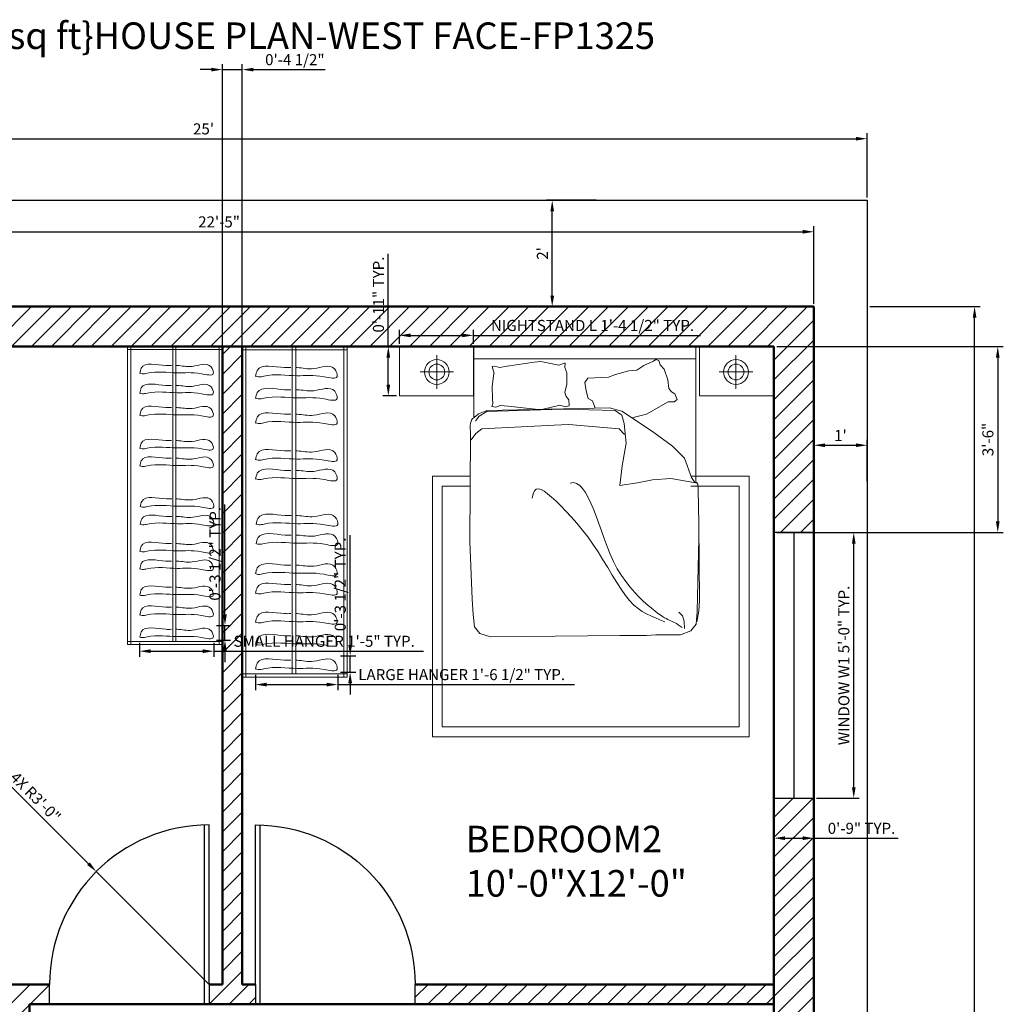
# Model space of a CAD drawing. Units: inches. Extents: x 3542 to 3908, y 2103 to 2666.
# Tile 4 of 4: x 3685 to 3907, y 2444 to 2666. Entities that reach past the tile are written whole.
import ezdxf

# ---------------------------------------------------------------- set-up
doc = ezdxf.new("R2010")
doc.units = ezdxf.units.IN
for name, color, linetype, lineweight in [('A-ANNO-DIMS', 2, 'Continuous', 18), ('A-ANNO-TEXT', 7, 'Continuous', 25), ('A-AREA-IDEN', 7, 'Continuous', 25), ('A-DOOR', 3, 'Continuous', 25), ('A-FLOR-CASE', 8, 'Continuous', 18), ('A-FURN', 8, 'Continuous', 18), ('A-GLAZ', 5, 'Continuous', 25), ('A-WALL', 7, 'Continuous', 50), ('A-WALL-PATT', 252, 'Continuous', 13), ('C-PROP', 7, 'Continuous', 25)]:
    doc.layers.add(name, color=color, linetype=linetype, lineweight=lineweight)
doc.styles.get("Standard").update_dxf_attribs({"font": 'arial.ttf'})
doc.dimstyles.new('ISO-25', dxfattribs={"dimtxt": 2.5, "dimasz": 2.5, "dimexe": 1.25, "dimexo": 0.625, "dimtad": 1, "dimdec": 0, "dimlunit": 3, "dimtxsty": 'Standard', "dimcen": 2.5, "dimadec": 0, "dimazin": 0, "dimtfac": 1, "dimtdec": 0, "dimtmove": 0, "dimatfit": 3, "dimfxl": 1, "dimarcsym": 0})

# ---------------------------------------------------------------- blocks, each defined once
blk = doc.blocks.new('*D5')
at = {"layer": 'A-ANNO-DIMS', "color": 0, "lineweight": -2, "transparency": 16777216}
for p, q in [((3815.51, 2625.48), (3804.33, 2625.48)), ((3805.58, 2603.98), (3805.58, 2622.98)), ((3815.51, 2601.48), (3804.33, 2601.48))]:
    blk.add_line(p, q, dxfattribs=at)
at = {"layer": 'A-ANNO-DIMS', "color": 0, "transparency": 16777216}
for points in [[(3805.17, 2622.98), (3806, 2622.98), (3805.58, 2625.48)], [(3805.17, 2603.98), (3806, 2603.98), (3805.58, 2601.48)]]:
    blk.add_solid(points, dxfattribs=at)
at = {"layer": 'Defpoints', "color": 0, "transparency": 16777216}
for p in [(3805.58, 2625.48), (3816.14, 2625.48), (3816.14, 2601.48)]:
    blk.add_point(p, dxfattribs=at)
at = {"layer": 'A-ANNO-DIMS', "color": 0, "transparency": 16777216, "insert": (3803.7, 2613.48), "char_height": 2.5, "attachment_point": 5, "rotation": 90}
blk.add_mtext("2'", dxfattribs=at)
blk = doc.blocks.new('*D6')
at = {"layer": 'A-ANNO-DIMS', "color": 0, "lineweight": -2, "transparency": 16777216}
for p, q in [((3864.64, 2562.06), (3864.64, 2571.43)), ((3867.14, 2570.18), (3874.14, 2570.18)), ((3876.64, 2562.06), (3876.64, 2571.43))]:
    blk.add_line(p, q, dxfattribs=at)
at = {"layer": 'A-ANNO-DIMS', "color": 0, "transparency": 16777216}
for points in [[(3867.14, 2570.6), (3867.14, 2569.77), (3864.64, 2570.18)], [(3874.14, 2570.6), (3874.14, 2569.77), (3876.64, 2570.18)]]:
    blk.add_solid(points, dxfattribs=at)
at = {"layer": 'Defpoints', "color": 0, "transparency": 16777216}
for p in [(3876.64, 2570.18), (3864.64, 2561.44), (3876.64, 2561.44)]:
    blk.add_point(p, dxfattribs=at)
at = {"layer": 'A-ANNO-DIMS', "color": 0, "transparency": 16777216, "insert": (3870.64, 2572.06), "char_height": 2.5, "attachment_point": 5}
blk.add_mtext("1'", dxfattribs=at)
blk = doc.blocks.new('*D8')
at = {"layer": 'A-ANNO-DIMS', "color": 0, "lineweight": -2, "transparency": 16777216}
for p, q in [((3596.14, 2602.1), (3596.14, 2619.62)), ((3598.64, 2618.37), (3862.14, 2618.37)), ((3864.64, 2602.1), (3864.64, 2619.62))]:
    blk.add_line(p, q, dxfattribs=at)
at = {"layer": 'A-ANNO-DIMS', "color": 0, "transparency": 16777216}
for points in [[(3598.64, 2618.79), (3598.64, 2617.96), (3596.14, 2618.37)], [(3862.14, 2618.79), (3862.14, 2617.96), (3864.64, 2618.37)]]:
    blk.add_solid(points, dxfattribs=at)
at = {"layer": 'Defpoints', "color": 0, "transparency": 16777216}
for p in [(3864.64, 2618.37), (3596.14, 2601.48), (3864.64, 2601.48)]:
    blk.add_point(p, dxfattribs=at)
at = {"layer": 'A-ANNO-DIMS', "color": 0, "transparency": 16777216, "insert": (3730.39, 2620.28), "char_height": 2.5, "attachment_point": 5}
blk.add_mtext('22\'-5"', dxfattribs=at)
blk = doc.blocks.new('*D9')
at = {"layer": 'A-ANNO-DIMS', "color": 0, "lineweight": -2, "transparency": 16777216}
for p, q in [((3577.14, 2626.1), (3577.14, 2640.63)), ((3876.64, 2626.1), (3876.64, 2640.63)), ((3579.64, 2639.38), (3874.14, 2639.38))]:
    blk.add_line(p, q, dxfattribs=at)
at = {"layer": 'A-ANNO-DIMS', "color": 0, "transparency": 16777216}
for points in [[(3579.64, 2639.8), (3579.64, 2638.96), (3577.14, 2639.38)], [(3874.14, 2639.8), (3874.14, 2638.96), (3876.64, 2639.38)]]:
    blk.add_solid(points, dxfattribs=at)
at = {"layer": 'Defpoints', "color": 0, "transparency": 16777216}
for p in [(3876.64, 2639.38), (3577.14, 2625.48), (3876.64, 2625.48)]:
    blk.add_point(p, dxfattribs=at)
at = {"layer": 'A-ANNO-DIMS', "color": 0, "transparency": 16777216, "insert": (3726.89, 2641.28), "char_height": 2.5, "attachment_point": 5}
blk.add_mtext("25'", dxfattribs=at)
blk = doc.blocks.new('*D11')
at = {"layer": 'A-ANNO-DIMS', "color": 0, "lineweight": -2, "transparency": 16777216}
for p, q in [((3877.27, 2601.48), (3902.16, 2601.48)), ((3900.91, 2208.98), (3900.91, 2598.98)), ((3877.27, 2206.48), (3902.16, 2206.48))]:
    blk.add_line(p, q, dxfattribs=at)
at = {"layer": 'A-ANNO-DIMS', "color": 0, "transparency": 16777216}
for points in [[(3900.5, 2598.98), (3901.33, 2598.98), (3900.91, 2601.48)], [(3900.5, 2208.98), (3901.33, 2208.98), (3900.91, 2206.48)]]:
    blk.add_solid(points, dxfattribs=at)
at = {"layer": 'Defpoints', "color": 0, "transparency": 16777216}
for p in [(3876.64, 2601.48), (3900.91, 2601.48), (3876.64, 2206.48)]:
    blk.add_point(p, dxfattribs=at)
at = {"layer": 'A-ANNO-DIMS', "color": 0, "transparency": 16777216, "insert": (3899.01, 2403.98), "char_height": 2.5, "attachment_point": 5, "rotation": 90}
blk.add_mtext('32\'-11"', dxfattribs=at)
blk = doc.blocks.new('DOOR-SWING-36IN')
for p, q in [((35, 0), (35, 40.5)), ((36, 4.5), (36, 40.5))]:
    blk.add_line(p, q)
blk.add_arc((36, 4.5), 36, 90, 180)
blk = doc.blocks.new('WIN-60IN')
for p, q in [((0, 60), (0, 0)), ((4.5, 60), (4.5, 0)), ((9, 0), (9, 60))]:
    blk.add_line(p, q)
blk = doc.blocks.new('NIGHTSTAND-LARGE')
for p, q in [((8.44, 9.16), (8.44, 1.59)), ((4.65, 5.38), (12.22, 5.38))]:
    blk.add_line(p, q)
blk.add_lwpolyline([(0, 0), (16.7, 0), (16.7, 11.13), (0, 11.13)], close=True)
for radius in [2.79, 1.78]:
    blk.add_circle((8.44, 5.38), radius)
blk = doc.blocks.new('WARDROBE-HANGER-S')
for points, knots in [([(8.24, 2.17), (8.32, 2.16), (9.48, 2.12), (12.01, 1.44), (15.78, 3.3), (17.2, -0.48), (12.35, 0.82), (8.34, 0.2), (3.56, 1.01), (0.75, 0.17), (0.19, 0.36), (0, 0.42)], [256.949798, 256.949798, 256.949798, 256.949798, 263.372126, 359.428036, 478.655159, 522.640662, 597.66786, 752.004169, 941.88133, 973.527729, 990.309099, 990.309099, 990.309099, 990.309099]), ([(0.04, 0.35), (0.12, 0.8), (0.56, 3.21), (4.46, 2.1), (6.78, 2.14), (7.18, 2.15)], [0, 0, 0, 0, 35.911014, 192.421107, 225.897258, 225.897258, 225.897258, 225.897258])]:
    blk.add_open_spline(points, degree=3, knots=knots)
blk = doc.blocks.new('WARDROBE-HANGER-L')
for points, knots in [([(9.15, 2.4), (9.23, 2.4), (10.51, 2.35), (13.33, 1.6), (17.51, 3.66), (19.09, -0.53), (13.7, 0.9), (9.26, 0.22), (3.95, 1.12), (0.83, 0.19), (0.21, 0.4), (0, 0.47)], [256.949798, 256.949798, 256.949798, 256.949798, 263.372126, 359.428036, 478.655159, 522.640662, 597.66786, 752.004169, 941.88133, 973.527729, 990.309099, 990.309099, 990.309099, 990.309099]), ([(0.04, 0.39), (0.13, 0.88), (0.62, 3.56), (4.95, 2.33), (7.52, 2.38), (7.96, 2.39)], [0, 0, 0, 0, 35.911014, 192.421107, 225.897258, 225.897258, 225.897258, 225.897258])]:
    blk.add_open_spline(points, degree=3, knots=knots)
blk = doc.blocks.new('*D24')
at = {"layer": 'A-ANNO-DIMS', "color": 0, "lineweight": -2, "transparency": 16777216}
for p, q in [((3712.45, 2525.58), (3712.45, 2522.44)), ((3729.21, 2525.58), (3729.21, 2522.44)), ((3714.95, 2523.69), (3726.71, 2523.69)), ((3729.21, 2523.69), (3776.52, 2523.69))]:
    blk.add_line(p, q, dxfattribs=at)
at = {"layer": 'A-ANNO-DIMS', "color": 0, "transparency": 16777216}
for points in [[(3714.95, 2524.11), (3714.95, 2523.28), (3712.45, 2523.69)], [(3726.71, 2524.11), (3726.71, 2523.28), (3729.21, 2523.69)]]:
    blk.add_solid(points, dxfattribs=at)
at = {"layer": 'Defpoints', "color": 0, "transparency": 16777216}
for p in [(3712.45, 2526.21), (3729.21, 2526.21), (3729.21, 2523.69)]:
    blk.add_point(p, dxfattribs=at)
at = {"layer": 'A-ANNO-DIMS', "color": 0, "transparency": 16777216, "insert": (3754.11, 2525.61), "char_height": 2.5, "attachment_point": 5}
blk.add_mtext('SMALL HANGER 1\'-5" TYP.', dxfattribs=at)
blk = doc.blocks.new('*D25')
at = {"layer": 'A-ANNO-DIMS', "color": 0, "lineweight": -2, "transparency": 16777216}
for p, q in [((3731.72, 2532.01), (3731.72, 2556.82)), ((3729.83, 2529.51), (3732.97, 2529.51)), ((3731.72, 2526.21), (3731.72, 2529.51)), ((3729.83, 2526.21), (3732.97, 2526.21)), ((3731.72, 2523.71), (3731.72, 2521.21))]:
    blk.add_line(p, q, dxfattribs=at)
at = {"layer": 'A-ANNO-DIMS', "color": 0, "transparency": 16777216}
for points in [[(3731.3, 2532.01), (3732.14, 2532.01), (3731.72, 2529.51)], [(3731.3, 2523.71), (3732.14, 2523.71), (3731.72, 2526.21)]]:
    blk.add_solid(points, dxfattribs=at)
at = {"layer": 'Defpoints', "color": 0, "transparency": 16777216}
for p in [(3729.21, 2529.51), (3731.72, 2529.51), (3729.21, 2526.21)]:
    blk.add_point(p, dxfattribs=at)
at = {"layer": 'A-ANNO-DIMS', "color": 0, "transparency": 16777216, "insert": (3729.8, 2545.67), "char_height": 2.5, "attachment_point": 5, "rotation": 90}
blk.add_mtext('0\'-3 1/2" TYP.', dxfattribs=at)
blk = doc.blocks.new('*D26')
at = {"layer": 'A-ANNO-DIMS', "color": 0, "lineweight": -2, "transparency": 16777216}
for p, q in [((3738.6, 2518.32), (3738.6, 2514.91)), ((3757.19, 2518.32), (3757.19, 2514.91)), ((3741.1, 2516.16), (3754.69, 2516.16)), ((3757.19, 2516.16), (3810.62, 2516.16))]:
    blk.add_line(p, q, dxfattribs=at)
at = {"layer": 'A-ANNO-DIMS', "color": 0, "transparency": 16777216}
for points in [[(3741.1, 2516.57), (3741.1, 2515.74), (3738.6, 2516.16)], [(3754.69, 2516.57), (3754.69, 2515.74), (3757.19, 2516.16)]]:
    blk.add_solid(points, dxfattribs=at)
at = {"layer": 'Defpoints', "color": 0, "transparency": 16777216}
for p in [(3738.6, 2518.95), (3757.19, 2518.95), (3757.19, 2516.16)]:
    blk.add_point(p, dxfattribs=at)
at = {"layer": 'A-ANNO-DIMS', "color": 0, "transparency": 16777216, "insert": (3785.15, 2518.08), "char_height": 2.5, "attachment_point": 5}
blk.add_mtext('LARGE HANGER 1\'-6 1/2" TYP.', dxfattribs=at)
blk = doc.blocks.new('*D27')
at = {"layer": 'A-ANNO-DIMS', "color": 0, "lineweight": -2, "transparency": 16777216}
for p, q in [((3759.98, 2525.11), (3759.98, 2549.92)), ((3757.82, 2522.61), (3761.23, 2522.61)), ((3759.98, 2518.95), (3759.98, 2522.61)), ((3757.82, 2518.95), (3761.23, 2518.95)), ((3759.98, 2516.45), (3759.98, 2513.95))]:
    blk.add_line(p, q, dxfattribs=at)
at = {"layer": 'A-ANNO-DIMS', "color": 0, "transparency": 16777216}
for points in [[(3759.56, 2525.11), (3760.4, 2525.11), (3759.98, 2522.61)], [(3759.56, 2516.45), (3760.4, 2516.45), (3759.98, 2518.95)]]:
    blk.add_solid(points, dxfattribs=at)
at = {"layer": 'Defpoints', "color": 0, "transparency": 16777216}
for p in [(3757.19, 2522.61), (3759.98, 2522.61), (3757.19, 2518.95)]:
    blk.add_point(p, dxfattribs=at)
at = {"layer": 'A-ANNO-DIMS', "color": 0, "transparency": 16777216, "insert": (3758.06, 2538.77), "char_height": 2.5, "attachment_point": 5, "rotation": 90}
blk.add_mtext('0\'-3 1/2" TYP.', dxfattribs=at)
blk = doc.blocks.new('*D30')
at = {"layer": 'A-ANNO-DIMS', "color": 0, "lineweight": -2, "transparency": 16777216}
for p, q in [((3865.27, 2550.48), (3874.89, 2550.48)), ((3873.64, 2492.98), (3873.64, 2547.98)), ((3865.27, 2490.48), (3874.89, 2490.48))]:
    blk.add_line(p, q, dxfattribs=at)
at = {"layer": 'A-ANNO-DIMS', "color": 0, "transparency": 16777216}
for points in [[(3873.23, 2547.98), (3874.06, 2547.98), (3873.64, 2550.48)], [(3873.23, 2492.98), (3874.06, 2492.98), (3873.64, 2490.48)]]:
    blk.add_solid(points, dxfattribs=at)
at = {"layer": 'Defpoints', "color": 0, "transparency": 16777216}
for p in [(3864.64, 2550.48), (3873.64, 2550.48), (3864.64, 2490.48)]:
    blk.add_point(p, dxfattribs=at)
at = {"layer": 'A-ANNO-DIMS', "color": 0, "transparency": 16777216, "insert": (3871.73, 2520.48), "char_height": 2.5, "attachment_point": 5, "rotation": 90}
blk.add_mtext('WINDOW W1 5\'-0" TYP.', dxfattribs=at)
blk = doc.blocks.new('*D31')
at = {"layer": 'A-ANNO-DIMS', "color": 0, "lineweight": -2, "transparency": 16777216}
for p, q in [((3855.64, 2489.85), (3855.64, 2480.23)), ((3864.64, 2489.85), (3864.64, 2480.23)), ((3858.14, 2481.48), (3862.14, 2481.48)), ((3864.64, 2481.48), (3883.63, 2481.48))]:
    blk.add_line(p, q, dxfattribs=at)
at = {"layer": 'A-ANNO-DIMS', "color": 0, "transparency": 16777216}
for points in [[(3858.14, 2481.9), (3858.14, 2481.06), (3855.64, 2481.48)], [(3862.14, 2481.9), (3862.14, 2481.06), (3864.64, 2481.48)]]:
    blk.add_solid(points, dxfattribs=at)
at = {"layer": 'Defpoints', "color": 0, "transparency": 16777216}
for p in [(3855.64, 2490.48), (3864.64, 2490.48), (3864.64, 2481.48)]:
    blk.add_point(p, dxfattribs=at)
at = {"layer": 'A-ANNO-DIMS', "color": 0, "transparency": 16777216, "insert": (3875.39, 2483.38), "char_height": 2.5, "attachment_point": 5}
blk.add_mtext('0\'-9" TYP.', dxfattribs=at)
blk = doc.blocks.new('*D36')
at = {"layer": 'A-ANNO-DIMS', "color": 0, "lineweight": -2, "transparency": 16777216}
for p, q in [((3771.1, 2593.1), (3771.1, 2596.23)), ((3787.8, 2593.1), (3787.8, 2596.23)), ((3773.6, 2594.98), (3785.3, 2594.98)), ((3787.8, 2594.98), (3839.07, 2594.98))]:
    blk.add_line(p, q, dxfattribs=at)
at = {"layer": 'A-ANNO-DIMS', "color": 0, "transparency": 16777216}
for points in [[(3773.6, 2595.4), (3773.6, 2594.57), (3771.1, 2594.98)], [(3785.3, 2595.4), (3785.3, 2594.57), (3787.8, 2594.98)]]:
    blk.add_solid(points, dxfattribs=at)
at = {"layer": 'Defpoints', "color": 0, "transparency": 16777216}
for p in [(3787.8, 2594.98), (3771.1, 2592.48), (3787.8, 2592.48)]:
    blk.add_point(p, dxfattribs=at)
at = {"layer": 'A-ANNO-DIMS', "color": 0, "transparency": 16777216, "insert": (3814.68, 2596.9), "char_height": 2.5, "attachment_point": 5}
blk.add_mtext('NIGHTSTAND L 1\'-4 1/2" TYP.', dxfattribs=at)
blk = doc.blocks.new('*D37')
at = {"layer": 'A-ANNO-DIMS', "color": 0, "lineweight": -2, "transparency": 16777216}
for p, q in [((3768.59, 2592.48), (3768.59, 2613.41)), ((3770.47, 2592.48), (3767.34, 2592.48)), ((3768.59, 2583.84), (3768.59, 2589.98)), ((3770.47, 2581.34), (3767.34, 2581.34))]:
    blk.add_line(p, q, dxfattribs=at)
at = {"layer": 'A-ANNO-DIMS', "color": 0, "transparency": 16777216}
for points in [[(3768.18, 2589.98), (3769.01, 2589.98), (3768.59, 2592.48)], [(3768.18, 2583.84), (3769.01, 2583.84), (3768.59, 2581.34)]]:
    blk.add_solid(points, dxfattribs=at)
at = {"layer": 'Defpoints', "color": 0, "transparency": 16777216}
for p in [(3768.59, 2592.48), (3771.1, 2592.48), (3771.1, 2581.34)]:
    blk.add_point(p, dxfattribs=at)
at = {"layer": 'A-ANNO-DIMS', "color": 0, "transparency": 16777216, "insert": (3766.69, 2604.19), "char_height": 2.5, "attachment_point": 5, "rotation": 90}
blk.add_mtext('0\'-11" TYP.', dxfattribs=at)
blk = doc.blocks.new('*D51')
at = {"layer": 'A-ANNO-DIMS', "color": 0, "lineweight": -2, "transparency": 16777216}
for p, q in [((3731.14, 2449.1), (3731.14, 2656.23)), ((3735.64, 2449.1), (3735.64, 2656.23)), ((3728.64, 2654.98), (3726.14, 2654.98)), ((3731.14, 2654.98), (3735.64, 2654.98)), ((3738.14, 2654.98), (3754.37, 2654.98))]:
    blk.add_line(p, q, dxfattribs=at)
at = {"layer": 'A-ANNO-DIMS', "color": 0, "transparency": 16777216}
for points in [[(3728.64, 2655.4), (3728.64, 2654.56), (3731.14, 2654.98)], [(3738.14, 2655.4), (3738.14, 2654.56), (3735.64, 2654.98)]]:
    blk.add_solid(points, dxfattribs=at)
at = {"layer": 'Defpoints', "color": 0, "transparency": 16777216}
for p in [(3735.64, 2654.98), (3731.14, 2448.48), (3735.64, 2448.48)]:
    blk.add_point(p, dxfattribs=at)
at = {"layer": 'A-ANNO-DIMS', "color": 0, "transparency": 16777216, "insert": (3747.5, 2656.9), "char_height": 2.5, "attachment_point": 5}
blk.add_mtext('0\'-4 1/2"', dxfattribs=at)
blk = doc.blocks.new('*D52')
at = {"layer": 'A-ANNO-DIMS', "color": 0, "lineweight": -2, "transparency": 16777216}
for p, q in [((3856.27, 2592.48), (3907.39, 2592.48)), ((3906.14, 2589.98), (3906.14, 2552.98)), ((3856.27, 2550.48), (3907.39, 2550.48))]:
    blk.add_line(p, q, dxfattribs=at)
at = {"layer": 'A-ANNO-DIMS', "color": 0, "transparency": 16777216}
for points in [[(3905.73, 2589.98), (3906.56, 2589.98), (3906.14, 2592.48)], [(3905.73, 2552.98), (3906.56, 2552.98), (3906.14, 2550.48)]]:
    blk.add_solid(points, dxfattribs=at)
at = {"layer": 'Defpoints', "color": 0, "transparency": 16777216}
for p in [(3855.64, 2592.48), (3855.64, 2550.48), (3906.14, 2550.48)]:
    blk.add_point(p, dxfattribs=at)
at = {"layer": 'A-ANNO-DIMS', "color": 0, "transparency": 16777216, "insert": (3904.24, 2571.48), "char_height": 2.5, "attachment_point": 5, "rotation": 90}
blk.add_mtext('3\'-6"', dxfattribs=at)
blk = doc.blocks.new('*D65')
at = {"layer": 'A-ANNO-DIMS', "color": 0, "lineweight": -2, "transparency": 16777216}
for p, q in [((3681.84, 2494.78), (3700.92, 2475.7)), ((3728.14, 2448.48), (3702.69, 2473.94))]:
    blk.add_line(p, q, dxfattribs=at)
at = {"layer": 'A-ANNO-DIMS', "color": 0, "transparency": 16777216}
blk.add_solid([(3701.22, 2476), (3700.63, 2475.41), (3702.69, 2473.94)], dxfattribs=at)
at = {"layer": 'Defpoints', "color": 0, "transparency": 16777216}
for p in [(3702.69, 2473.94), (3728.14, 2448.48)]:
    blk.add_point(p, dxfattribs=at)
at = {"layer": 'A-ANNO-DIMS', "color": 0, "transparency": 16777216, "insert": (3688.76, 2490.55), "char_height": 2.5, "attachment_point": 5, "rotation": 314.9996}
blk.add_mtext('4X R3\'-0"', dxfattribs=at)

msp = doc.modelspace()

# ---------------------------------------------------------------- hatches: boundary and pattern name
at = {"layer": 'A-WALL-PATT'}
h = msp.add_hatch(dxfattribs=at)
h.set_pattern_fill('ANSI31', color=256)
h.paths.add_polyline_path([(3864.64, 2601.48), (3596.14, 2601.48), (3596.14, 2550.48), (3605.14, 2550.48), (3605.14, 2592.48), (3855.64, 2592.48), (3855.64, 2550.48), (3864.64, 2550.48)])
h.paths.add_polyline_path([(3735.64, 2592.48), (3731.14, 2592.48), (3731.14, 2448.48), (3728.14, 2448.48), (3728.14, 2443.98), (3738.64, 2443.98), (3738.64, 2448.48), (3735.64, 2448.48)])
h.paths.add_polyline_path([(3855.64, 2448.48), (3774.64, 2448.48), (3774.64, 2443.98), (3855.64, 2443.98)])
h.paths.add_polyline_path([(3605.14, 2490.48), (3596.14, 2490.48), (3596.14, 2426.98), (3605.14, 2426.98)])
h.paths.add_polyline_path([(3605.14, 2402.98), (3596.14, 2402.98), (3596.14, 2350.98), (3605.14, 2350.98)])
h.paths.add_polyline_path([(3692.14, 2448.48), (3605.14, 2448.48), (3605.14, 2443.98), (3683.14, 2443.98), (3683.14, 2440.98), (3687.64, 2440.98), (3687.64, 2443.98), (3692.14, 2443.98)])
h.paths.add_polyline_path([(3687.64, 2404.98), (3683.14, 2404.98), (3683.14, 2385.98), (3605.14, 2385.98), (3605.14, 2381.48), (3687.64, 2381.48)])
h.paths.add_polyline_path([(3864.64, 2490.48), (3855.64, 2490.48), (3855.64, 2397.98), (3864.64, 2397.98)])
h.paths.add_polyline_path([(3864.64, 2337.98), (3855.64, 2337.98), (3855.64, 2269.48), (3864.64, 2269.48)])
h.paths.add_polyline_path([(3864.64, 2233.48), (3855.64, 2233.48), (3855.64, 2215.48), (3831.64, 2215.48), (3831.64, 2206.48), (3864.64, 2206.48)])
h.paths.add_polyline_path([(3771.64, 2215.48), (3740.31, 2215.48), (3740.31, 2206.48), (3771.64, 2206.48)])
h.paths.add_polyline_path([(3747.64, 2287.48), (3750.64, 2287.48), (3750.64, 2291.98), (3743.14, 2291.98), (3743.14, 2215.48), (3747.64, 2215.48)])
h.paths.add_polyline_path([(3706.76, 2215.48), (3695.14, 2215.48), (3695.14, 2291.98), (3690.64, 2291.98), (3690.64, 2206.48), (3690.64, 2158.48), (3665.89, 2158.48), (3665.89, 2153.98), (3690.64, 2153.98), (3699.64, 2153.98), (3699.64, 2206.48), (3706.76, 2206.48)])
h.paths.add_polyline_path([(3605.14, 2314.98), (3596.14, 2314.98), (3596.14, 2153.98), (3629.89, 2153.98), (3629.89, 2158.48), (3605.14, 2158.48)])

# ---------------------------------------------------------------- linework, layer by layer
at = {"layer": 'A-DOOR'}
for p, q in [((3692.14, 2443.98), (3692.14, 2448.48)), ((3728.14, 2448.48), (3728.14, 2443.98)), ((3738.64, 2448.48), (3738.64, 2443.98)), ((3774.64, 2443.98), (3774.64, 2448.48))]:
    msp.add_line(p, q, dxfattribs=at)
at = {"layer": 'A-FLOR-CASE'}
for p, q in [((3709.76, 2592.48), (3709.76, 2525.19)), ((3709.76, 2592.48), (3731.14, 2592.48)), ((3709.76, 2591.77), (3731.14, 2591.77)), ((3710.47, 2592.48), (3710.47, 2525.19)), ((3719.95, 2592.48), (3719.95, 2525.9)), ((3720.66, 2592.48), (3720.66, 2525.9)), ((3730.43, 2525.19), (3730.43, 2592.48)), ((3731.14, 2525.19), (3731.14, 2592.48)), ((3735.61, 2592.48), (3735.61, 2517.81)), ((3735.61, 2592.48), (3759.34, 2592.48)), ((3735.61, 2591.69), (3759.34, 2591.69)), ((3736.4, 2592.48), (3736.4, 2517.81)), ((3746.92, 2592.48), (3746.92, 2518.61)), ((3747.71, 2592.48), (3747.71, 2518.61)), ((3758.55, 2517.81), (3758.55, 2592.48)), ((3759.34, 2517.81), (3759.34, 2592.48)), ((3709.76, 2525.9), (3731.14, 2525.9)), ((3709.76, 2525.19), (3731.14, 2525.19)), ((3735.61, 2518.61), (3759.34, 2518.61)), ((3735.61, 2517.81), (3759.34, 2517.81))]:
    msp.add_line(p, q, dxfattribs=at)
at = {"layer": 'A-FURN'}
for p, q in [((3787.86, 2576.37), (3787.86, 2592.48)), ((3792.47, 2586.35), (3792.04, 2587.97)), ((3803, 2589.11), (3801.48, 2588.94)), ((3807.11, 2588.25), (3803, 2589.11)), ((3808.37, 2588.72), (3807.11, 2588.25)), ((3808.49, 2588.68), (3808.37, 2588.72)), ((3808.49, 2588.68), (3808.4, 2587.75)), ((3808.49, 2588.68), (3808.4, 2587.75)), ((3808.4, 2587.75), (3808.9, 2586.54)), ((3824.67, 2587.12), (3826.23, 2588.16)), ((3824.67, 2587.12), (3826.23, 2588.16)), ((3826.23, 2588.16), (3828.44, 2589.19)), ((3829.94, 2588.33), (3830.83, 2587.36)), ((3830.83, 2587.36), (3831.67, 2584.94)), ((3808.9, 2586.54), (3808.88, 2583.98)), ((3813.59, 2585.29), (3818.3, 2585.56)), ((3818.3, 2585.56), (3819.89, 2586.17)), ((3819.89, 2586.17), (3822.9, 2586.98)), ((3822.9, 2586.98), (3824.67, 2587.12)), ((3808.88, 2583.98), (3808.42, 2582.08)), ((3831.67, 2584.94), (3831.88, 2583)), ((3831.88, 2583), (3832.49, 2582.25)), ((3808.42, 2582.08), (3808.74, 2581.18)), ((3808.74, 2581.18), (3809.3, 2580.45)), ((3832.49, 2582.25), (3833.26, 2581.76)), ((3833.26, 2581.76), (3833.79, 2580.53)), ((3807.31, 2579.26), (3803.24, 2578.23)), ((3808.59, 2578.86), (3807.31, 2579.26)), ((3809.38, 2579.11), (3808.59, 2578.86)), ((3809.3, 2580.45), (3809.38, 2579.11)), ((3831.79, 2579.97), (3826.85, 2577.2)), ((3833.13, 2580.02), (3831.79, 2579.97)), ((3833.79, 2580.53), (3833.13, 2580.02)), ((3787.15, 2575.27), (3787.08, 2574.49)), ((3787.08, 2574.49), (3787.11, 2572.67)), ((3787.11, 2572.67), (3787, 2548.42)), ((3837.89, 2561.73), (3837.99, 2561.78)), ((3838.64, 2552.4), (3838.56, 2560.27)), ((3838.81, 2535.17), (3838.64, 2552.4)), ((3787, 2548.42), (3787.53, 2535.41)), ((3838.69, 2549.02), (3838.35, 2536.01)), ((3787.53, 2535.41), (3787.71, 2532.01)), ((3838.35, 2536.01), (3838.28, 2532.6)), ((3838.67, 2532.78), (3838.81, 2535.17)), ((3787.71, 2532.01), (3788.01, 2529.2)), ((3834.97, 2531.64), (3834.16, 2532.49)), ((3838.28, 2532.6), (3838.06, 2529.79)), ((3838.2, 2530.3), (3838.67, 2532.78)), ((3835.35, 2530.5), (3834.97, 2531.64)), ((3835.42, 2528.84), (3835.35, 2530.5)), ((3838.06, 2529.79), (3836.88, 2528.26)), ((3788.01, 2529.2), (3789.24, 2527.72)), ((3789.24, 2527.72), (3791.62, 2526.92)), ((3820.86, 2527.24), (3791.62, 2526.92)), ((3820.86, 2527.24), (3826.83, 2527.24)), ((3826.83, 2527.24), (3828.95, 2527.39)), ((3828.95, 2527.39), (3834.53, 2527.39)), ((3836.88, 2528.26), (3834.53, 2527.39))]:
    msp.add_line(p, q, dxfattribs=at)
for points in [[(3787.86, 2592.48), (3837.98, 2592.48), (3837.98, 2561.82)], [(3837.98, 2589.7), (3787.86, 2589.7)], [(3829.94, 2588.33), (3829.62, 2589.35), (3828.96, 2589.56), (3828.44, 2589.19)], [(3801.48, 2588.94), (3795.42, 2588.03), (3793.67, 2587.73), (3792.62, 2588.07), (3792.04, 2587.97)], [(3801.72, 2578.33), (3795.62, 2578.97), (3793.86, 2579.18), (3792.83, 2578.8), (3791.97, 2578.91), (3792.21, 2579.58), (3792.07, 2580.74), (3792.03, 2583.42), (3792.41, 2586.35)], [(3813.59, 2585.29), (3812.95, 2584.36), (3813.25, 2582.43), (3813.72, 2580.72), (3814.65, 2580.18), (3815.19, 2578.79), (3815.19, 2578.53)], [(3788.28, 2576.67), (3788.97, 2577.27), (3790.84, 2578.05), (3818.53, 2578.6), (3821.31, 2577.88), (3825.76, 2574.93), (3828.55, 2573.08), (3832.75, 2570), (3835.43, 2567.27), (3837.01, 2562.89), (3837.79, 2561.74)], [(3787.18, 2575.31), (3787.34, 2575.84), (3787.58, 2576.24), (3787.86, 2576.37), (3788.19, 2576.66), (3788.23, 2576.68)], [(3837.98, 2561.71), (3832.36, 2562.69), (3828.21, 2562.38), (3824.83, 2561.7), (3820.81, 2561.13), (3821.35, 2565.52), (3822.25, 2570.62), (3821.86, 2575.12), (3821.27, 2576.94), (3819.8, 2577.99), (3807.92, 2578.31), (3790.85, 2577.8), (3789.1, 2576.77), (3788.36, 2575.75), (3788.27, 2575.65)], [(3826.85, 2577.2), (3823.56, 2576.39)], [(3821.92, 2572.63), (3820.66, 2573.91), (3809.36, 2574.87), (3806.06, 2574.68), (3789.7, 2573.86), (3788.32, 2572.82), (3787.28, 2571.43)], [(3836.9, 2563.2), (3850, 2563.2), (3850, 2504.36), (3778.55, 2504.36), (3778.55, 2563.2), (3787.07, 2563.2)], [(3836.9, 2560.98), (3847.77, 2560.98), (3847.77, 2506.59), (3780.78, 2506.59), (3780.78, 2560.98), (3787.07, 2560.98)], [(3834.93, 2529.02), (3834.46, 2529.37), (3834.04, 2529.67), (3833.65, 2529.91), (3833.3, 2530.11), (3832.96, 2530.28), (3832.64, 2530.43), (3832.32, 2530.57), (3831.99, 2530.71), (3831.66, 2530.87), (3831.3, 2531.05), (3830.9, 2531.26), (3830.46, 2531.53), (3829.95, 2531.87), (3829.38, 2532.28), (3828.73, 2532.78), (3827.98, 2533.38), (3827.14, 2534.1), (3826.21, 2534.94), (3825.23, 2535.89), (3824.21, 2536.95), (3823.18, 2538.12), (3822.17, 2539.41), (3821.19, 2540.81), (3820.27, 2542.31), (3819.43, 2543.92), (3818.66, 2545.61), (3817.96, 2547.34), (3817.3, 2549.1), (3816.68, 2550.84), (3816.08, 2552.55), (3815.5, 2554.19), (3814.91, 2555.73), (3814.32, 2557.14), (3813.72, 2558.41), (3813.1, 2559.51), (3812.45, 2560.41), (3811.79, 2561.1), (3811.09, 2561.56), (3810.36, 2561.75), (3809.6, 2561.66)], [(3838.55, 2560.34), (3838.48, 2561.43), (3838.16, 2561.75), (3837.98, 2561.82)], [(3830.97, 2530.33), (3829.91, 2530.8), (3828.87, 2531.23), (3827.86, 2531.66), (3826.88, 2532.12), (3825.91, 2532.66), (3824.95, 2533.31), (3824, 2534.11), (3823.04, 2535.1), (3822.09, 2536.29), (3821.12, 2537.67), (3820.14, 2539.2), (3819.13, 2540.84), (3818.1, 2542.56), (3817.04, 2544.32), (3815.93, 2546.09), (3814.78, 2547.83), (3813.59, 2549.5), (3812.36, 2551.1), (3811.12, 2552.61), (3809.89, 2554.03), (3808.69, 2555.33), (3807.53, 2556.52), (3806.44, 2557.57), (3805.44, 2558.49), (3804.54, 2559.25), (3803.75, 2559.83), (3803.06, 2560.22), (3802.47, 2560.37), (3801.97, 2560.28), (3801.58, 2559.91), (3801.29, 2559.23), (3801.08, 2558.24)]]:
    msp.add_lwpolyline(points, dxfattribs=at)
at = {"layer": 'A-GLAZ'}
for p, q in [((3864.64, 2550.48), (3855.64, 2550.48)), ((3855.64, 2490.48), (3864.64, 2490.48))]:
    msp.add_line(p, q, dxfattribs=at)
at = {"layer": 'A-WALL'}
for p, q in [((3596.14, 2601.48), (3864.64, 2601.48)), ((3596.14, 2601.48), (3864.64, 2601.48)), ((3864.64, 2601.48), (3864.64, 2206.48)), ((3605.14, 2592.48), (3855.64, 2592.48)), ((3731.14, 2592.48), (3731.14, 2448.48)), ((3735.64, 2592.48), (3735.64, 2448.48)), ((3855.64, 2592.48), (3855.64, 2215.48)), ((3605.14, 2448.48), (3692.14, 2448.48)), ((3728.14, 2448.48), (3731.14, 2448.48)), ((3735.64, 2448.48), (3738.64, 2448.48)), ((3774.64, 2448.48), (3855.64, 2448.48)), ((3687.64, 2443.98), (3687.64, 2381.48)), ((3687.64, 2443.98), (3731.14, 2443.98)), ((3695.14, 2443.98), (3855.64, 2443.98))]:
    msp.add_line(p, q, dxfattribs=at)
at = {"layer": 'C-PROP'}
for p, q in [((3596.14, 2625.48), (3864.64, 2625.48)), ((3864.64, 2625.48), (3876.64, 2625.48)), ((3876.64, 2625.48), (3876.64, 2601.48)), ((3876.64, 2601.48), (3876.64, 2206.48))]:
    msp.add_line(p, q, dxfattribs=at)

# ---------------------------------------------------------------- block references
at = {"layer": 'A-DOOR'}
msp.add_blockref('DOOR-SWING-36IN', (3692.14, 2443.98), dxfattribs=at)
at = {"layer": 'A-DOOR', "extrusion": (0, 0, -1), "zscale": -1}
msp.add_blockref('DOOR-SWING-36IN', (-3774.64, 2443.98), dxfattribs=at)
at = {"layer": 'A-FLOR-CASE'}
for name, p in [('WARDROBE-HANGER-S', (3712.45, 2586.03)), ('WARDROBE-HANGER-L', (3738.6, 2585.32)), ('WARDROBE-HANGER-S', (3712.45, 2581.53)), ('WARDROBE-HANGER-L', (3738.6, 2580.33)), ('WARDROBE-HANGER-S', (3712.45, 2576.54)), ('WARDROBE-HANGER-L', (3738.6, 2574.79)), ('WARDROBE-HANGER-S', (3712.45, 2569.08)), ('WARDROBE-HANGER-L', (3738.6, 2566.51)), ('WARDROBE-HANGER-S', (3712.45, 2565.11)), ('WARDROBE-HANGER-L', (3738.6, 2562.12)), ('WARDROBE-HANGER-S', (3712.56, 2555.92)), ('WARDROBE-HANGER-S', (3712.56, 2551.96)), ('WARDROBE-HANGER-L', (3738.72, 2551.92)), ('WARDROBE-HANGER-L', (3738.72, 2547.52)), ('WARDROBE-HANGER-S', (3712.45, 2545.84)), ('WARDROBE-HANGER-S', (3712.45, 2541.88)), ('WARDROBE-HANGER-L', (3738.6, 2540.73)), ('WARDROBE-HANGER-S', (3712.45, 2535.97)), ('WARDROBE-HANGER-L', (3738.6, 2536.33)), ('WARDROBE-HANGER-S', (3712.45, 2531.47)), ('WARDROBE-HANGER-L', (3738.6, 2529.78)), ('WARDROBE-HANGER-S', (3712.45, 2526.48)), ('WARDROBE-HANGER-L', (3738.6, 2524.79)), ('WARDROBE-HANGER-L', (3738.6, 2519.25))]:
    msp.add_blockref(name, p, dxfattribs=at)
at = {"layer": 'A-FURN'}
msp.add_blockref('NIGHTSTAND-LARGE', (3771.1, 2581.34), dxfattribs=at)
at = {"layer": 'A-FURN', "extrusion": (0, 0, -1), "zscale": -1}
msp.add_blockref('NIGHTSTAND-LARGE', (-3855.5, 2581.34), dxfattribs=at)
at = {"layer": 'A-GLAZ'}
msp.add_blockref('WIN-60IN', (3855.64, 2490.48), dxfattribs=at)

# ---------------------------------------------------------------- texts
at = {"layer": 'A-ANNO-TEXT', "insert": (3637.21, 2665.63), "char_height": 6, "width": 219.7452, "attachment_point": 1}
msp.add_mtext('25X40\\{1000 sq ft\\}HOUSE PLAN-WEST FACE-FP1325', dxfattribs=at)
at = {"layer": 'A-AREA-IDEN', "insert": (3786.05, 2484.28), "char_height": 6, "attachment_point": 1}
msp.add_mtext('BEDROOM2\\P10\'-0"X12\'-0"', dxfattribs=at)

# ---------------------------------------------------------------- dimensions: what is measured, and where the dimension line sits
at = {"layer": 'A-ANNO-DIMS'}
for base, p1, p2, override, picture, middle in [((3735.64, 2654.98), (3731.14, 2448.48), (3735.64, 2448.48), {"dimdec": 1, "dimlfac": 1, "dimrnd": 0, "dimzin": 1, "dimdsep": 46, "dimlunit": 4, "dimfrac": 2}, '*D51', (3747.5, 2656.9)), ((3876.64448065, 2639.37837652), (3577.14448065, 2625.47915136), (3876.64448065, 2625.47915136), {"dimclrd": 0, "dimclre": 0, "dimclrt": 0}, '*D9', (3726.89448065, 2641.27980899)), ((3864.64448065, 2618.37377621), (3596.14448065, 2601.47915136), (3864.64448065, 2601.47915136), {"dimclrd": 0, "dimclre": 0, "dimclrt": 0}, '*D8', (3730.39448065, 2620.27520868)), ((3876.64, 2570.18), (3864.64, 2561.44), (3876.64, 2561.44), {"dimclrd": 0, "dimclre": 0, "dimclrt": 0}, '*D6', (3870.64, 2572.06))]:
    dim = msp.add_linear_dim(base=base, p1=p1, p2=p2, dimstyle='ISO-25', override=override, dxfattribs=at)
    dim.commit()
    dim.dimension.update_dxf_attribs({"geometry": picture, "text_midpoint": middle})
for base, p1, p2, override, picture, middle in [((3805.58, 2625.48), (3816.14, 2601.48), (3816.14, 2625.48), {"dimclrd": 0, "dimclre": 0, "dimclrt": 0}, '*D5', (3803.7, 2613.48)), ((3900.91, 2601.48), (3876.64, 2206.48), (3876.64, 2601.48), {"dimclrd": 0, "dimclre": 0, "dimclrt": 0}, '*D11', (3899.01, 2403.98)), ((3906.14, 2550.48), (3855.64, 2592.48), (3855.64, 2550.48), {"dimdec": 1, "dimlfac": 1, "dimrnd": 0, "dimzin": 1, "dimdsep": 46, "dimlunit": 4, "dimfrac": 2}, '*D52', (3904.24, 2571.48))]:
    dim = msp.add_linear_dim(base=base, p1=p1, p2=p2, angle=90, dimstyle='ISO-25', override=override, dxfattribs=at)
    dim.commit()
    dim.dimension.update_dxf_attribs({"geometry": picture, "text_midpoint": middle})
for base, p1, p2, text, picture, middle in [((3768.59, 2592.48), (3771.1, 2581.34), (3771.1, 2592.48), '<> TYP.', '*D37', (3766.69, 2604.19)), ((3731.72, 2529.51), (3729.21, 2526.21), (3729.21, 2529.51), '<> TYP.', '*D25', (3729.8, 2545.67)), ((3759.98, 2522.61), (3757.19, 2518.95), (3757.19, 2522.61), '<> TYP.', '*D27', (3758.06, 2538.77)), ((3873.64, 2550.48), (3864.64, 2490.48), (3864.64, 2550.48), 'WINDOW W1 <> TYP.', '*D30', (3871.73, 2520.48))]:
    dim = msp.add_linear_dim(base=base, p1=p1, p2=p2, angle=90, text=text, dimstyle='ISO-25', override={"dimdec": 1, "dimlfac": 1, "dimrnd": 0, "dimzin": 1, "dimdsep": 46, "dimlunit": 4, "dimfrac": 2}, dxfattribs=at)
    dim.commit()
    dim.dimension.update_dxf_attribs({"geometry": picture, "text_midpoint": middle})
for base, p1, p2, text, picture, middle in [((3787.8, 2594.98), (3771.1, 2592.48), (3787.8, 2592.48), 'NIGHTSTAND L <> TYP.', '*D36', (3814.68, 2596.9)), ((3729.21, 2523.69), (3712.45, 2526.21), (3729.21, 2526.21), 'SMALL HANGER <> TYP.', '*D24', (3754.11, 2525.61)), ((3757.19, 2516.16), (3738.6, 2518.95), (3757.19, 2518.95), 'LARGE HANGER <> TYP.', '*D26', (3785.15, 2518.08)), ((3864.64, 2481.48), (3855.64, 2490.48), (3864.64, 2490.48), '<> TYP.', '*D31', (3875.39, 2483.38))]:
    dim = msp.add_linear_dim(base=base, p1=p1, p2=p2, text=text, dimstyle='ISO-25', override={"dimdec": 1, "dimlfac": 1, "dimrnd": 0, "dimzin": 1, "dimdsep": 46, "dimlunit": 4, "dimfrac": 2}, dxfattribs=at)
    dim.commit()
    dim.dimension.update_dxf_attribs({"geometry": picture, "text_midpoint": middle})
dim = msp.add_radius_dim(center=(3728.14, 2448.48), mpoint=(3702.69, 2473.94), text='4X <>', dimstyle='ISO-25', override={"dimdec": 1, "dimlfac": 1, "dimrnd": 0, "dimzin": 1, "dimdsep": 46, "dimlunit": 4, "dimfrac": 2}, dxfattribs=at)
dim.commit()
dim.dimension.update_dxf_attribs({"geometry": '*D65', "text_midpoint": (3687.42, 2489.21), "dimtype": 164})

doc.saveas('drawing.dxf')
